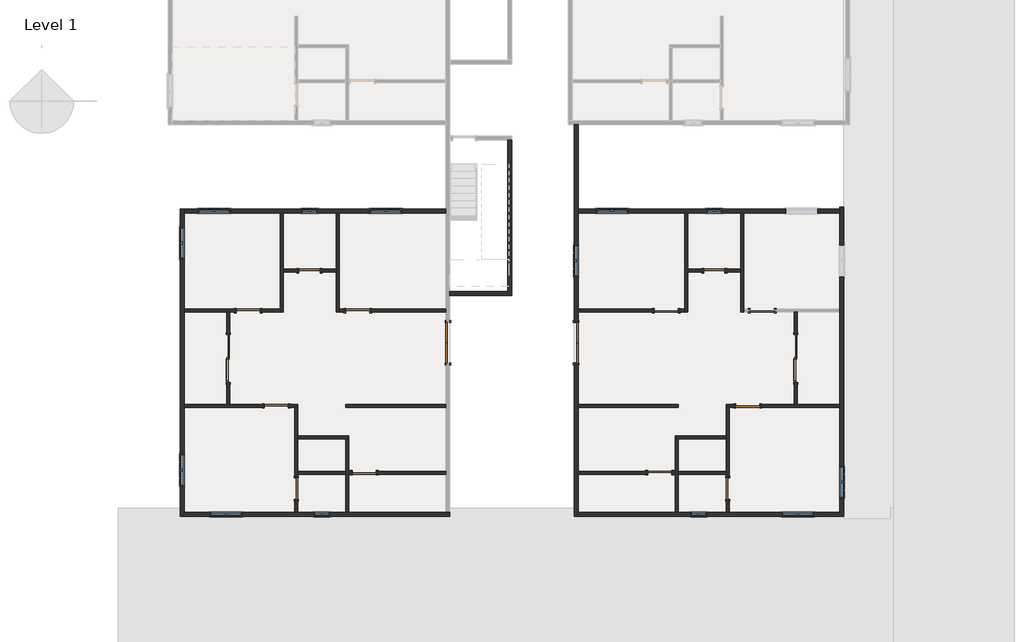
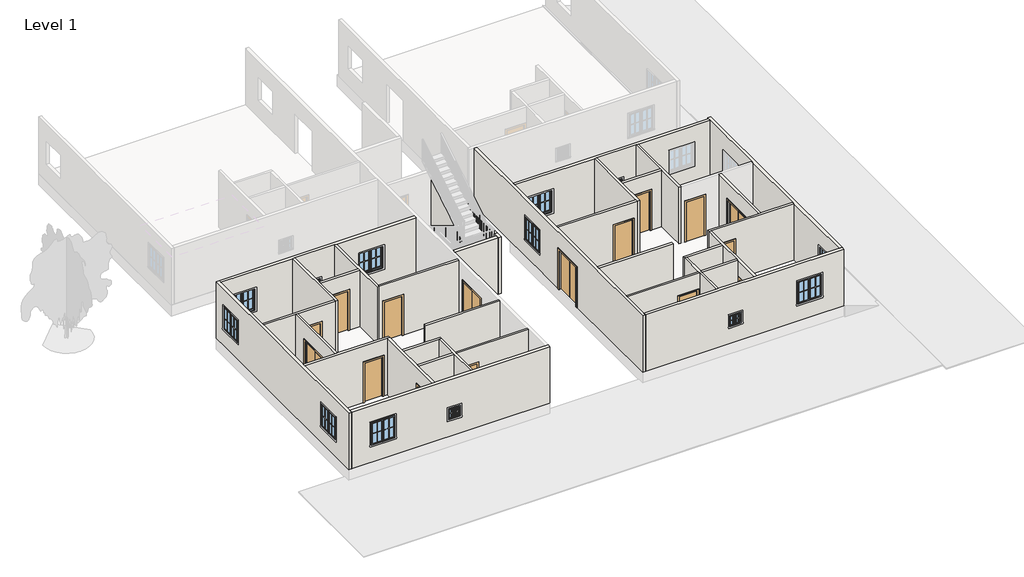
# One storey, part 1 of 7: 32 walls, 16 doors, 13 windows.
# Revit data of these elements (continued)
# Element 53 (IfcWindow, "Window-Casement-Double : 48\" x 48\"") (continued)
#   Interior Wall Closure = 0' - 2 1/4"
#   Frame Extension = 0' - 0 1/4"
#   Exterior Wall Closure = 0' - 1 1/4"
#   Interior Trim Visibility = yes
#   Exterior Trim Visibility = yes
#   Phase Created = New Construction
#   Materials on its faces: "Wood - Stained", "Glass", "Clad - White"
# Element 54 (IfcWindow, "Window-Casement-Double : 48\" x 48\"")
#   Mark = "13"
#   Window Inset = 0' - 0"
#   Interior Wall Closure = 0' - 2 1/4"
#   Frame Extension = 0' - 0 1/4"
#   Exterior Wall Closure = 0' - 1 1/4"
#   Interior Trim Visibility = yes
#   Exterior Trim Visibility = yes
#   Phase Created = New Construction
#   Materials on its faces: "Wood - Stained", "Glass", "Clad - White"
# Element 55 (IfcWindow, "Window-Casement-Double : 48\" x 48\"")
#   Mark = "14"
#   Window Inset = 0' - 0"
#   Interior Wall Closure = 0' - 2 1/4"
#   Frame Extension = 0' - 0 1/4"
#   Exterior Wall Closure = 0' - 1 1/4"
#   Interior Trim Visibility = yes
#   Exterior Trim Visibility = yes
#   Phase Created = New Construction
#   Materials on its faces: "Wood - Stained", "Glass", "Clad - White"
# Element 56 (IfcWindow, "Window-Casement-Double : 48\" x 48\"")
#   Mark = "15"
#   Window Inset = 0' - 0"
#   Interior Wall Closure = 0' - 2 1/4"
#   Frame Extension = 0' - 0 1/4"
#   Exterior Wall Closure = 0' - 1 1/4"
#   Interior Trim Visibility = yes
#   Exterior Trim Visibility = yes
#   Phase Created = New Construction
#   Materials on its faces: "Wood - Stained", "Glass", "Clad - White"
# Element 57 (IfcWindow, "Window-Casement-Double : 48\" x 48\"")
#   Mark = "16"
#   Window Inset = 0' - 0"
#   Interior Wall Closure = 0' - 2 1/4"
#   Frame Extension = 0' - 0 1/4"
#   Exterior Wall Closure = 0' - 1 1/4"
#   Interior Trim Visibility = yes
#   Exterior Trim Visibility = yes
#   Phase Created = New Construction
#   Materials on its faces: "Wood - Stained", "Glass", "Clad - White"
# Element 58 (IfcWindow, "Window-Casement-Double : 48\" x 48\"")
#   Mark = "17"
#   Window Inset = 0' - 0"
#   Interior Wall Closure = 0' - 2 1/4"
#   Frame Extension = 0' - 0 1/4"
#   Exterior Wall Closure = 0' - 1 1/4"
#   Interior Trim Visibility = yes
#   Exterior Trim Visibility = yes
#   Phase Created = New Construction
#   Materials on its faces: "Wood - Stained", "Glass", "Clad - White"
# Element 59 (IfcWindow, "Window-Casement-Double : 48\" x 48\"")
#   Mark = "18"
#   Window Inset = 0' - 0"
#   Interior Wall Closure = 0' - 2 1/4"
#   Frame Extension = 0' - 0 1/4"
#   Exterior Wall Closure = 0' - 1 1/4"
#   Interior Trim Visibility = yes
#   Exterior Trim Visibility = yes
#   Phase Created = New Construction
#   Materials on its faces: "Wood - Stained", "Glass", "Clad - White"
# Element 60 (IfcWindow, "Window-Casement-Double : 48\" x 48\"")
#   Mark = "21"
#   Window Inset = 0' - 0"
#   Interior Wall Closure = 0' - 2 1/4"
#   Frame Extension = 0' - 0 1/4"
#   Exterior Wall Closure = 0' - 1 1/4"
#   Interior Trim Visibility = yes
#   Exterior Trim Visibility = yes
#   Phase Created = New Construction
#   Materials on its faces: "Wood - Stained", "Glass", "Clad - White"
# Element 61 (IfcWindow, "Window-Casement-Double : 48\" x 48\"")
#   Mark = "22"
#   Window Inset = 0' - 0"
#   Interior Wall Closure = 0' - 2 1/4"
#   Frame Extension = 0' - 0 1/4"
#   Exterior Wall Closure = 0' - 1 1/4"
#   Interior Trim Visibility = yes
#   Exterior Trim Visibility = yes
#   Phase Created = New Construction
#   Materials on its faces: "Wood - Stained", "Glass", "Clad - White"
# Materials
#   "Wood - Birch - Solid Stained Light Low Gloss": class "Wood", colour RGB 210 159 95, transparency 0, Cost = 0
#   "Paint - Sienna": colour RGB 118 70 51, transparency 0, Cost = 0
#   "Glass": class "Glass", colour RGB 0 128 192, transparency 0.75, Description = "Soda Lime Glass", Cost = 0
#   "Door - Panel": class "Wood", colour RGB 210 159 95, transparency 0, Cost = 0
#   "Door - Frame": colour RGB 118 70 51, transparency 0, Cost = 0
#   "4.5\" WALL": class "Generic", colour RGB 120 120 120, transparency 0, Cost = 0
#   "6\" WALL": class "Generic", colour RGB 120 120 120, transparency 0, Cost = 0
#   "Wood - Stained": class "Wood", colour RGB 224 178 126, transparency 0, Cost = 0
#   "Clad - White": class "Wood", colour RGB 242 242 238, transparency 0, Cost = 0
